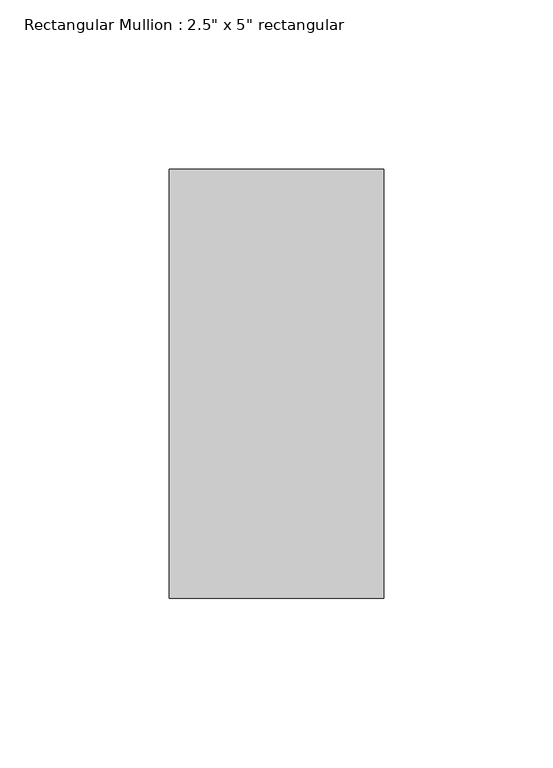
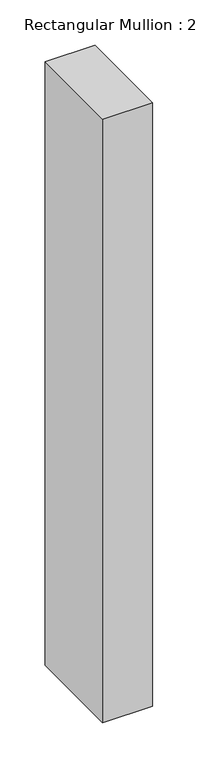
"""IFC4 building model written with IfcOpenShell, lengths in millimetres: member geometry."""

from ifc_helpers import new_model, si_unit, frame, origin, place, context, project, spatial, polyline, outline, extrude, source, transform, mapped, element, save


def member_58a4a87b(model_context):
    return source(origin(), model_context, "Body", "SweptSolid", [
        extrude(outline(polyline([(31.75, 63.5), (31.75, -63.5), (-31.75, -63.5), (-31.75, 63.5), (31.75, 63.5)])), frame((0.0, 0.0, -812.8), z_axis=(0.0, 0.0, 1.0), x_axis=(1.0, 0.0, 0.0)), (0.0, 0.0, 1.0), 812.8),
    ])


if __name__ == "__main__":
    model = new_model("IFC4")
    model_context = context("Model", 3, world=origin())
    ifc_project = project(units=[si_unit("LENGTHUNIT", "METRE", prefix="MILLI")], contexts=[model_context])
    site = spatial("IfcSite", under=ifc_project)
    building = spatial("IfcBuilding", under=site)
    placement = place(None, origin())
    member_shape = member_58a4a87b(model_context)
    element("IfcMember", 1, ObjectType="Rectangular Mullion : 2.5\" x 5\" rectangular", at=placement, inside=building, context=model_context, shape_type="MappedRepresentation", body=[
        mapped(member_shape, transform((0.0, 0.0, 0.0), x_axis=(1.0, 0.0, 0.0), y_axis=(0.0, 1.0, 0.0), z_axis=(0.0, 0.0, 1.0))),
    ])
    save(model, "model.ifc")

# Revit data of these elements
# Type "Rectangular Mullion : 2.5\" x 5\" rectangular"
#   built-in parameter 1007304 = 0.416667 (stored number, unit not read)
#   built-in parameter 1007301 = 0.104167 (stored number, unit not read)
#   built-in parameter 1007300 = 0.104167 (stored number, unit not read)
# Element 1 (IfcMember, "Rectangular Mullion : 2.5\" x 5\" rectangular")
#   Materials on its faces: "Aluminum"
# Materials
#   "Aluminum": class "Metal", colour RGB 247 247 247, transparency 0, Description = "Aluminum 6061", Cost = 0
